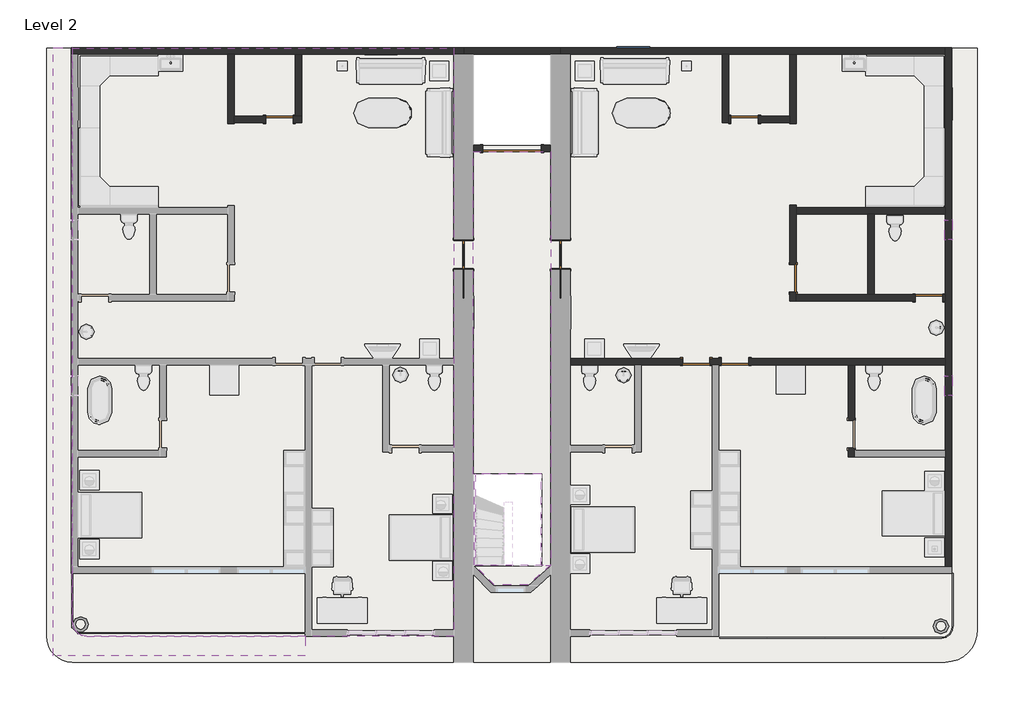
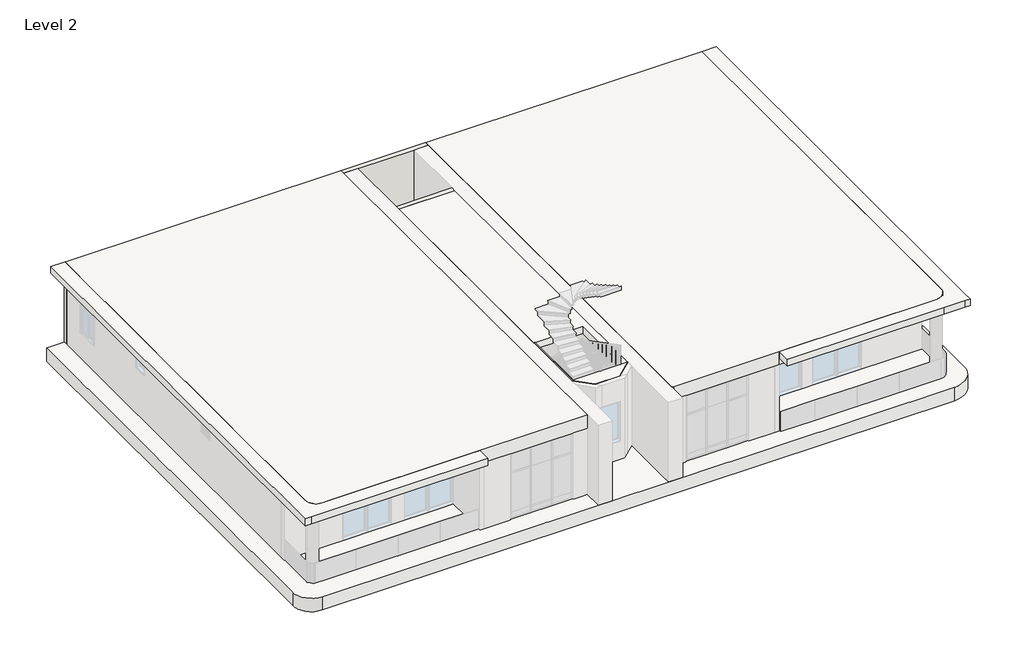
# One storey, part 3 of 5: 17 walls, 9 doors, 5 windows, 4 slabs, 1 roof.
"""IFC4 building model written with IfcOpenShell, lengths in millimetres."""

from ifc_helpers import new_model, si_unit, point, frame, frame_2d, origin, place, context, project, spatial, polyline, circle_curve, trimmed, segment, composite_curve, outline, extrude, faceted_brep, transform, mapped, element, save
from components import door_4726f842, door_ede55593, door_2703ae13, door_10fd3a06, window_0038ecf3, window_54100e87

model = new_model("IFC4")

# Units and contexts
model_context = context("Model", 3, world=origin())
ifc_project = project(units=[si_unit("LENGTHUNIT", "METRE", prefix="MILLI")], contexts=[model_context])

# Site, building, storey
site = spatial("IfcSite", under=ifc_project)
building = spatial("IfcBuilding", under=site)
storey = spatial("IfcBuildingStorey", under=building, Name="Level 2", Elevation=3657.6)

# Doors
placement = place(None, origin())
door_shape = door_4726f842(model_context)
element("IfcDoor", 1, ObjectType="Door-Double-Flush_Panel-Double-Acting : 72\" x 84\"", at=placement, inside=storey, context=model_context, shape_type="MappedRepresentation", body=[
    mapped(door_shape, transform((-4793.1987704, 8549.6758558, 3657.6), x_axis=(-1.0, 0.0, 0.0), y_axis=(0.0, -1.0, 0.0), z_axis=(0.0, 0.0, 1.0))),
])
door_2_shape = door_ede55593(model_context)
element("IfcDoor", 2, ObjectType="Door-Interior-Single-Pocket-2_Panel-Wood : 36\" x 96\"", at=placement, inside=storey, context=model_context, shape_type="MappedRepresentation", body=[
    mapped(door_2_shape, transform((-6317.1987704, 5196.8758558, 3657.6), x_axis=(0.0, -1.0, 0.0), y_axis=(1.0, 0.0, 0.0), z_axis=(0.0, 0.0, 1.0))),
])
element("IfcDoor", 3, ObjectType="Door-Interior-Single-Pocket-2_Panel-Wood : 36\" x 96\"", at=placement, inside=storey, context=model_context, shape_type="MappedRepresentation", body=[
    mapped(door_2_shape, transform((-3269.1987704, 5196.8758558, 3657.6), x_axis=(0.0, -1.0, 0.0), y_axis=(1.0, 0.0, 0.0), z_axis=(0.0, 0.0, 1.0))),
])
door_3_shape = door_2703ae13(model_context)
element("IfcDoor", 4, ObjectType="Door-Single-Panel.0001 : 34\" x 80\"", at=placement, inside=storey, context=model_context, shape_type="MappedRepresentation", body=[
    mapped(door_3_shape, transform((998.0012296, 1844.0758558, 3657.6), x_axis=(1.0, 0.0, 0.0), y_axis=(0.0, 1.0, 0.0), z_axis=(0.0, 0.0, 1.0))),
])
element("IfcDoor", 5, ObjectType="Door-Single-Panel.0001 : 34\" x 80\"", at=placement, inside=storey, context=model_context, shape_type="MappedRepresentation", body=[
    mapped(door_3_shape, transform((2522.0012296, 9464.0758558, 3657.6), x_axis=(-1.0, 0.0, 0.0), y_axis=(0.0, -1.0, 0.0), z_axis=(0.0, 0.0, 1.0))),
])
door_4_shape = door_10fd3a06(model_context)
element("IfcDoor", 6, ObjectType="Door-Single-Panel.0001 : 34\" x 80\"", at=placement, inside=storey, context=model_context, shape_type="MappedRepresentation", body=[
    mapped(door_4_shape, transform((-12108.3987704, 9464.0758558, 3657.6), x_axis=(1.0, 0.0, 0.0), y_axis=(0.0, 1.0, 0.0), z_axis=(0.0, 0.0, 1.0))),
])
element("IfcDoor", 7, ObjectType="Door-Single-Panel.0001 : 34\" x 80\"", at=placement, inside=storey, context=model_context, shape_type="MappedRepresentation", body=[
    mapped(door_4_shape, transform((2217.2012296, 1844.0758558, 3657.6), x_axis=(-1.0, 0.0, 0.0), y_axis=(0.0, -1.0, 0.0), z_axis=(0.0, 0.0, 1.0))),
])
element("IfcDoor", 8, ObjectType="Door-Single-Panel.0001 : 34\" x 80\"", at=placement, inside=storey, context=model_context, shape_type="MappedRepresentation", body=[
    mapped(door_4_shape, transform((8313.2012296, 3850.6758558, 3657.6), x_axis=(1.0, 0.0, 0.0), y_axis=(0.0, 1.0, 0.0), z_axis=(0.0, 0.0, 1.0))),
])
element("IfcDoor", 9, ObjectType="Door-Single-Panel.0001 : 34\" x 80\"", at=placement, inside=storey, context=model_context, shape_type="MappedRepresentation", body=[
    mapped(door_4_shape, transform((4046.0012296, 4460.2758558, 3657.6), x_axis=(0.0, -1.0, 0.0), y_axis=(1.0, 0.0, 0.0), z_axis=(0.0, 0.0, 1.0))),
])

# Roof
element("IfcRoof", 10, ObjectType="Generic - 2' white 2", at=placement, inside=storey, context=model_context, shape_type="SweptSolid", body=[
    extrude(outline(composite_curve([segment(polyline([(-19423.5987704, 11699.2758558), (9837.2012296, 11699.2758558), (9837.2012296, -6588.7241442)]), True, "CONTINUOUS"), segment(trimmed(circle_curve(frame_2d((8821.2012296, -6588.7241442)), 1016.0), [point((9837.2012296, -6588.7241442))], [point((8821.2012296, -7604.7241442))], False, "CARTESIAN"), True, "CONTINUOUS"), segment(polyline([(8821.2012296, -7604.7241442), (-18610.7987704, -7604.7241442)]), True, "CONTINUOUS"), segment(trimmed(circle_curve(frame_2d((-18610.7987704, -6791.9241442)), 812.8), [point((-18610.7987704, -7604.7241442))], [point((-19423.5987704, -6791.9241442))], False, "CARTESIAN"), True, "CONTINUOUS"), segment(polyline([(-19423.5987704, -6791.9241442), (-19423.5987704, 11699.2758558)]), True, "CONTINUOUS")], self_intersect=False), holes=[polyline([(-6012.3987704, -4575.7741442), (-3853.3987704, -4575.7741442), (-3853.3987704, -1686.5241442), (-6012.3987704, -1686.5241442), (-6012.3987704, -4575.7741442)]), polyline([(-6012.3987704, 8651.2758558), (-3573.9987704, 8651.2758558), (-3573.9987704, 11521.4758558), (-6012.3987704, 11521.4758558), (-6012.3987704, 8651.2758558)])]), frame((0.0, 0.0, 3048.0), z_axis=(0.0, 0.0, 1.0), x_axis=(1.0, 0.0, 0.0)), (0.0, 0.0, 1.0), 609.6),
])

# Slabs
element("IfcSlab", 11, ObjectType="Generic - 12\" cream", at=placement, inside=storey, context=model_context, shape_type="SweptSolid", body=[
    extrude(outline(composite_curve([segment(polyline([(-6621.9987704, 11699.2758558), (-6621.9987704, -6791.9241442), (-11295.5987704, -6791.9241442), (-18153.5987704, -6791.9241442)]), True, "CONTINUOUS"), segment(trimmed(circle_curve(frame_2d((-18153.5987704, -6334.7241442)), 457.2), [point((-18153.5987704, -6791.9241442))], [point((-18610.7987704, -6334.7241442))], False, "CARTESIAN"), True, "CONTINUOUS"), segment(polyline([(-18610.7987704, -6334.7241442), (-18610.7987704, 11699.2758558), (-6621.9987704, 11699.2758558)]), True, "CONTINUOUS")], self_intersect=False)), frame((0.0, 0.0, 6705.6), z_axis=(0.0, 0.0, 1.0), x_axis=(1.0, 0.0, 0.0)), (0.0, 0.0, 1.0), 609.6),
    extrude(outline(composite_curve([segment(trimmed(circle_curve(frame_2d((8511.8043381, -6277.3874522)), 514.536692), [point((9024.4012296, -6322.0241442))], [point((8511.8043381, -6791.9241442))], False, "CARTESIAN"), True, "CONTINUOUS"), segment(polyline([(8511.8043381, -6791.9241442), (1709.2012296, -6791.9241442), (-2862.7987704, -6791.9241442), (-2964.3987704, -6791.9241442), (-2964.3987704, 11699.2758558), (9024.4012296, 11699.2758558), (9024.4012296, -6322.0241442)]), True, "CONTINUOUS")], self_intersect=False)), frame((0.0, 0.0, 6705.6), z_axis=(0.0, 0.0, 1.0), x_axis=(1.0, 0.0, 0.0)), (0.0, 0.0, 1.0), 609.6),
])
element("IfcSlab", 12, ObjectType="Generic - 12\" white", at=placement, inside=storey, context=model_context, shape_type="SweptSolid", body=[
    extrude(outline(composite_curve([segment(polyline([(9634.0012296, 11699.2758558), (9634.0012296, -6931.6241442), (9634.0012296, -7401.5241442), (9430.8012296, -7401.5241442), (8511.8043381, -7401.5241442), (1709.2012296, -7401.5241442), (1709.2012296, -6791.9241442), (8511.8043381, -6791.9241442)]), True, "CONTINUOUS"), segment(trimmed(circle_curve(frame_2d((8511.8043381, -6277.3874522)), 514.536692), [point((8511.8043381, -6791.9241442))], [point((9024.4012296, -6322.0241442))], True, "CARTESIAN"), True, "CONTINUOUS"), segment(polyline([(9024.4012296, -6322.0241442), (9024.4012296, 11699.2758558), (9634.0012296, 11699.2758558)]), True, "CONTINUOUS")], self_intersect=False)), frame((0.0, 0.0, 7010.4), z_axis=(0.0, 0.0, 1.0), x_axis=(1.0, 0.0, 0.0)), (0.0, 0.0, 1.0), 304.8),
    extrude(outline(composite_curve([segment(polyline([(-18610.7987704, 11724.6758558), (-18610.7987704, -6334.7241442)]), True, "CONTINUOUS"), segment(trimmed(circle_curve(frame_2d((-18153.5987704, -6334.7241442)), 457.2), [point((-18610.7987704, -6334.7241442))], [point((-18153.5987704, -6791.9241442))], True, "CARTESIAN"), True, "CONTINUOUS"), segment(polyline([(-18153.5987704, -6791.9241442), (-11295.5987704, -6791.9241442), (-11295.5987704, -7401.5241442), (-18966.3987704, -7401.5241442), (-19220.3987704, -7401.5241442), (-19220.3987704, 11724.6758558), (-18610.7987704, 11724.6758558)]), True, "CONTINUOUS")], self_intersect=False)), frame((0.0, 0.0, 7010.4), z_axis=(0.0, 0.0, 1.0), x_axis=(1.0, 0.0, 0.0)), (0.0, 0.0, 1.0), 304.8),
])
element("IfcSlab", 13, ObjectType="Generic - 12\" white", at=placement, inside=storey, context=model_context, shape_type="SweptSolid", body=[
    extrude(outline(polyline([(-3573.9987704, 8448.0758558), (-3573.9987704, -1691.5549149), (-3573.9987704, -4572.9908503), (-3878.7987704, -4572.9908503), (-3878.7987704, -1691.5549149), (-6012.3987704, -1691.5549149), (-6012.3987704, 8448.0758558), (-3573.9987704, 8448.0758558)])), frame((0.0, 0.0, 7010.4), z_axis=(0.0, 0.0, 1.0), x_axis=(1.0, 0.0, 0.0)), (0.0, 0.0, 1.0), 304.8),
])
element("IfcSlab", 14, ObjectType="Generic - 12\" white", at=placement, inside=storey, context=model_context, shape_type="SweptSolid", body=[
    extrude(outline(polyline([(-5940.8822214, -1691.5549149), (-5940.8822214, -4554.2130548), (-3578.6822214, -4554.2130548), (-4280.0806614, -5179.7242605), (-5346.8806614, -5179.7242605), (-5975.4985898, -4551.106332), (-5975.4985898, -1691.5549149), (-5940.8822214, -1691.5549149)])), frame((0.0, 0.0, 7010.4), z_axis=(0.0, 0.0, 1.0), x_axis=(1.0, 0.0, 0.0)), (0.0, 0.0, 1.0), 304.8),
])

# Walls
element("IfcWall", 15, ObjectType="Generic - 8\" cream", at=placement, inside=storey, context=model_context, shape_type="Brep", body=[
    faceted_brep([(-18648.8987704, 11521.4758558, 3657.6), (-18445.6987704, 11521.4758558, 3657.6), (-13733.9987704, 11521.4758558, 3657.6), (-13530.7987704, 11521.4758558, 3657.6), (-11600.3987704, 11521.4758558, 3657.6), (-11397.1987704, 11521.4758558, 3657.6), (-6621.9987704, 11521.4758558, 3657.6), (-6317.1987704, 11521.4758558, 3657.6), (-6317.1987704, 11521.4758558, 6705.6), (-6621.9987704, 11521.4758558, 6705.6), (-11397.1987704, 11521.4758558, 6705.6), (-11600.3987704, 11521.4758558, 6705.6), (-13530.7987704, 11521.4758558, 6705.6), (-13733.9987704, 11521.4758558, 6705.6), (-18445.6987704, 11521.4758558, 6705.6), (-18648.8987704, 11521.4758558, 6705.6), (-8450.7987704, 11521.4758558, 6096.0), (-8450.7987704, 11521.4758558, 4876.8), (-9365.1987704, 11521.4758558, 4876.8), (-9365.1987704, 11521.4758558, 6096.0), (-6317.1987704, 11724.6758558, 3657.6), (-18648.8987704, 11724.6758558, 3657.6), (-18648.8987704, 11724.6758558, 6705.6), (-6621.9987704, 11724.6758558, 6705.6), (-6317.1987704, 11724.6758558, 6705.6), (-8450.7987704, 11724.6758558, 4876.8), (-8450.7987704, 11724.6758558, 6096.0), (-9365.1987704, 11724.6758558, 6096.0), (-9365.1987704, 11724.6758558, 4876.8)], [[[0, 1, 2, 3, 4, 5, 6, 7, 8, 9, 10, 11, 12, 13, 14, 15], [16, 17, 18, 19]], [[20, 21, 22, 23, 24], [25, 26, 27, 28]], [[7, 6, 5, 4, 3, 2, 1, 0, 21, 20]], [[8, 7, 20, 24]], [[15, 14, 13, 12, 11, 10, 9, 8, 24, 23, 22]], [[0, 15, 22, 21]], [[16, 26, 25, 17]], [[17, 25, 28, 18]], [[18, 28, 27, 19]], [[26, 16, 19, 27]]]),
])
element("IfcWall", 16, ObjectType="Generic - 8\" cream", at=placement, inside=storey, context=model_context, shape_type="Brep", body=[
    faceted_brep([(8821.2012296, 11724.6758558, 3657.6), (8821.2012296, 11521.4758558, 3657.6), (8821.2012296, 6695.4758558, 3657.6), (8821.2012296, 6492.2758558, 3657.6), (8821.2012296, 3952.2758558, 3657.6), (8821.2012296, 3749.0758558, 3657.6), (8821.2012296, 1945.6758558, 3657.6), (8821.2012296, 1742.4758558, 3657.6), (8821.2012296, -949.9241442, 3657.6), (8821.2012296, -1153.1241442, 3657.6), (8821.2012296, -4607.5241442, 3657.6), (8821.2012296, -4607.5241442, 6705.6), (8821.2012296, -1153.1241442, 6705.6), (8821.2012296, -949.9241442, 6705.6), (8821.2012296, 1742.4758558, 6705.6), (8821.2012296, 1945.6758558, 6705.6), (8821.2012296, 3749.0758558, 6705.6), (8821.2012296, 3952.2758558, 6705.6), (8821.2012296, 6492.2758558, 6705.6), (8821.2012296, 6695.4758558, 6705.6), (8821.2012296, 11521.4758558, 6705.6), (8821.2012296, 11724.6758558, 6705.6), (8821.2012296, 10403.8758558, 4876.8), (8821.2012296, 10403.8758558, 6096.0), (8821.2012296, 9489.4758558, 6096.0), (8821.2012296, 9489.4758558, 4876.8), (8821.2012296, 777.2758558, 6400.8), (8821.2012296, 777.2758558, 5791.2), (8821.2012296, 1386.8758558, 5791.2), (8821.2012296, 1386.8758558, 6400.8), (8821.2012296, 6289.0758558, 5791.2), (8821.2012296, 6289.0758558, 6400.8), (8821.2012296, 5679.4758558, 6400.8), (8821.2012296, 5679.4758558, 5791.2), (9024.4012296, -4607.5241442, 3657.6), (9024.4012296, 11724.6758558, 3657.6), (9024.4012296, 11724.6758558, 6705.6), (9024.4012296, -4607.5241442, 6705.6), (9024.4012296, 10403.8758558, 6096.0), (9024.4012296, 10403.8758558, 4876.8), (9024.4012296, 9489.4758558, 4876.8), (9024.4012296, 9489.4758558, 6096.0), (9024.4012296, 777.2758558, 5791.2), (9024.4012296, 777.2758558, 6400.8), (9024.4012296, 1386.8758558, 6400.8), (9024.4012296, 1386.8758558, 5791.2), (9024.4012296, 6289.0758558, 6400.8), (9024.4012296, 6289.0758558, 5791.2), (9024.4012296, 5679.4758558, 5791.2), (9024.4012296, 5679.4758558, 6400.8)], [[[0, 1, 2, 3, 4, 5, 6, 7, 8, 9, 10, 11, 12, 13, 14, 15, 16, 17, 18, 19, 20, 21], [22, 23, 24, 25], [26, 27, 28, 29], [30, 31, 32, 33]], [[34, 35, 36, 37], [38, 39, 40, 41], [42, 43, 44, 45], [46, 47, 48, 49]], [[10, 9, 8, 7, 6, 5, 4, 3, 2, 1, 0, 35, 34]], [[21, 20, 19, 18, 17, 16, 15, 14, 13, 12, 11, 37, 36]], [[0, 21, 36, 35]], [[11, 10, 34, 37]], [[39, 38, 23, 22]], [[40, 39, 22, 25]], [[41, 40, 25, 24]], [[38, 41, 24, 23]], [[26, 43, 42, 27]], [[27, 42, 45, 28]], [[28, 45, 44, 29]], [[43, 26, 29, 44]], [[46, 31, 30, 47]], [[47, 30, 33, 48]], [[48, 33, 32, 49]], [[31, 46, 49, 32]]]),
])
element("IfcWall", 17, ObjectType="Generic - 8\" cream", at=placement, inside=storey, context=model_context, shape_type="Brep", body=[
    faceted_brep([(8821.2012296, 1742.4758558, 6705.6), (5976.4012296, 1742.4758558, 6705.6), (5773.2012296, 1742.4758558, 6705.6), (1709.2012296, 1742.4758558, 6705.6), (1506.0012296, 1742.4758558, 6705.6), (-729.1987704, 1742.4758558, 6705.6), (-932.3987704, 1742.4758558, 6705.6), (-2964.3987704, 1742.4758558, 6705.6), (-2964.3987704, 1742.4758558, 3657.6), (-932.3987704, 1742.4758558, 3657.6), (-729.1987704, 1742.4758558, 3657.6), (566.2012296, 1742.4758558, 3657.6), (566.2012296, 1742.4758558, 5689.6), (1429.8012296, 1742.4758558, 5689.6), (1429.8012296, 1742.4758558, 3657.6), (1506.0012296, 1742.4758558, 3657.6), (1709.2012296, 1742.4758558, 3657.6), (1785.4012296, 1742.4758558, 3657.6), (1785.4012296, 1742.4758558, 5689.6), (2649.0012296, 1742.4758558, 5689.6), (2649.0012296, 1742.4758558, 3657.6), (5773.2012296, 1742.4758558, 3657.6), (5976.4012296, 1742.4758558, 3657.6), (8821.2012296, 1742.4758558, 3657.6), (-2964.3987704, 1945.6758558, 6705.6), (8821.2012296, 1945.6758558, 6705.6), (8821.2012296, 1945.6758558, 3657.6), (2649.0012296, 1945.6758558, 3657.6), (2649.0012296, 1945.6758558, 5689.6), (1785.4012296, 1945.6758558, 5689.6), (1785.4012296, 1945.6758558, 3657.6), (1429.8012296, 1945.6758558, 3657.6), (1429.8012296, 1945.6758558, 5689.6), (566.2012296, 1945.6758558, 5689.6), (566.2012296, 1945.6758558, 3657.6), (-2964.3987704, 1945.6758558, 3657.6)], [[[0, 1, 2, 3, 4, 5, 6, 7, 8, 9, 10, 11, 12, 13, 14, 15, 16, 17, 18, 19, 20, 21, 22, 23]], [[24, 25, 26, 27, 28, 29, 30, 31, 32, 33, 34, 35]], [[8, 35, 34, 11, 10, 9]], [[26, 23, 22, 21, 20, 27]], [[14, 31, 30, 17, 16, 15]], [[7, 6, 5, 4, 3, 2, 1, 0, 25, 24]], [[0, 23, 26, 25]], [[8, 7, 24, 35]], [[13, 32, 31, 14]], [[32, 13, 12, 33]], [[33, 12, 11, 34]], [[29, 18, 17, 30]], [[18, 29, 28, 19]], [[19, 28, 27, 20]]]),
])
element("IfcWall", 18, ObjectType="Generic - 8\" cream", at=placement, inside=storey, context=model_context, shape_type="Brep", body=[
    faceted_brep([(-13733.9987704, 11521.4758558, 3657.6), (-13733.9987704, 9337.0758558, 3657.6), (-13733.9987704, 9337.0758558, 6705.6), (-13733.9987704, 11521.4758558, 6705.6), (-13530.7987704, 11521.4758558, 3657.6), (-13530.7987704, 11521.4758558, 6705.6), (-13530.7987704, 9565.6758558, 6705.6), (-13530.7987704, 9362.4758558, 6705.6), (-13530.7987704, 9337.0758558, 6705.6), (-13530.7987704, 9337.0758558, 3657.6), (-13530.7987704, 9362.4758558, 3657.6), (-13530.7987704, 9565.6758558, 3657.6)], [[[0, 1, 2, 3]], [[4, 5, 6, 7, 8, 9, 10, 11]], [[1, 0, 4, 11, 10, 9]], [[2, 1, 9, 8]], [[3, 2, 8, 7, 6, 5]], [[0, 3, 5, 4]]]),
])
element("IfcWall", 19, ObjectType="Generic - 8\" cream", at=placement, inside=storey, context=model_context, shape_type="Brep", body=[
    faceted_brep([(-11397.1987704, 9362.4758558, 6705.6), (-13530.7987704, 9362.4758558, 6705.6), (-13530.7987704, 9362.4758558, 3657.6), (-12540.1987704, 9362.4758558, 3657.6), (-12540.1987704, 9362.4758558, 5689.6), (-11676.5987704, 9362.4758558, 5689.6), (-11676.5987704, 9362.4758558, 3657.6), (-11397.1987704, 9362.4758558, 3657.6), (-13530.7987704, 9565.6758558, 6705.6), (-11600.3987704, 9565.6758558, 6705.6), (-11397.1987704, 9565.6758558, 6705.6), (-11397.1987704, 9565.6758558, 3657.6), (-11600.3987704, 9565.6758558, 3657.6), (-11676.5987704, 9565.6758558, 3657.6), (-11676.5987704, 9565.6758558, 5689.6), (-12540.1987704, 9565.6758558, 5689.6), (-12540.1987704, 9565.6758558, 3657.6), (-13530.7987704, 9565.6758558, 3657.6)], [[[0, 1, 2, 3, 4, 5, 6, 7]], [[8, 9, 10, 11, 12, 13, 14, 15, 16, 17]], [[2, 17, 16, 3]], [[11, 7, 6, 13, 12]], [[1, 0, 10, 9, 8]], [[2, 1, 8, 17]], [[0, 7, 11, 10]], [[5, 14, 13, 6]], [[14, 5, 4, 15]], [[15, 4, 3, 16]]]),
])
element("IfcWall", 20, ObjectType="Generic - 8\" cream", at=placement, inside=storey, context=model_context, shape_type="SweptSolid", body=[
    extrude(outline(polyline([(-11397.1987704, 11521.4758558), (-11397.1987704, 9565.6758558), (-11600.3987704, 9565.6758558), (-11600.3987704, 11521.4758558), (-11397.1987704, 11521.4758558)])), frame((0.0, 0.0, 3657.6), z_axis=(0.0, 0.0, 1.0), x_axis=(1.0, 0.0, 0.0)), (0.0, 0.0, 1.0), 3048.0),
])
element("IfcWall", 21, ObjectType="Generic - 8\" cream", at=placement, inside=storey, context=model_context, shape_type="Brep", body=[
    faceted_brep([(3944.4012296, 11521.4758558, 3657.6), (3944.4012296, 9565.6758558, 3657.6), (3944.4012296, 9362.4758558, 3657.6), (3944.4012296, 9337.0758558, 3657.6), (3944.4012296, 9337.0758558, 6705.6), (3944.4012296, 9362.4758558, 6705.6), (3944.4012296, 9565.6758558, 6705.6), (3944.4012296, 11521.4758558, 6705.6), (4147.6012296, 11521.4758558, 3657.6), (4147.6012296, 11521.4758558, 6705.6), (4147.6012296, 9337.0758558, 6705.6), (4147.6012296, 9337.0758558, 3657.6)], [[[0, 1, 2, 3, 4, 5, 6, 7]], [[8, 9, 10, 11]], [[3, 2, 1, 0, 8, 11]], [[4, 3, 11, 10]], [[7, 6, 5, 4, 10, 9]], [[0, 7, 9, 8]]]),
])
element("IfcWall", 22, ObjectType="Generic - 8\" cream", at=placement, inside=storey, context=model_context, shape_type="Brep", body=[
    faceted_brep([(4147.6012296, 6492.2758558, 3657.6), (6382.8012296, 6492.2758558, 3657.6), (6586.0012296, 6492.2758558, 3657.6), (8821.2012296, 6492.2758558, 3657.6), (8821.2012296, 6492.2758558, 6705.6), (6586.0012296, 6492.2758558, 6705.6), (6382.8012296, 6492.2758558, 6705.6), (4147.6012296, 6492.2758558, 6705.6), (4147.6012296, 6695.4758558, 3657.6), (4147.6012296, 6695.4758558, 6705.6), (8821.2012296, 6695.4758558, 6705.6), (8821.2012296, 6695.4758558, 3657.6)], [[[0, 1, 2, 3, 4, 5, 6, 7]], [[8, 9, 10, 11]], [[3, 2, 1, 0, 8, 11]], [[7, 6, 5, 4, 10, 9]], [[0, 7, 9, 8]], [[4, 3, 11, 10]]]),
])
element("IfcWall", 23, ObjectType="Generic - 8\" cream", at=placement, inside=storey, context=model_context, shape_type="Brep", body=[
    faceted_brep([(8821.2012296, 3749.0758558, 6705.6), (4147.6012296, 3749.0758558, 6705.6), (4147.6012296, 3749.0758558, 3657.6), (7881.4012296, 3749.0758558, 3657.6), (7881.4012296, 3749.0758558, 5689.6), (8745.0012296, 3749.0758558, 5689.6), (8745.0012296, 3749.0758558, 3657.6), (8821.2012296, 3749.0758558, 3657.6), (4147.6012296, 3952.2758558, 6705.6), (6382.8012296, 3952.2758558, 6705.6), (6586.0012296, 3952.2758558, 6705.6), (8821.2012296, 3952.2758558, 6705.6), (8821.2012296, 3952.2758558, 3657.6), (8745.0012296, 3952.2758558, 3657.6), (8745.0012296, 3952.2758558, 5689.6), (7881.4012296, 3952.2758558, 5689.6), (7881.4012296, 3952.2758558, 3657.6), (6586.0012296, 3952.2758558, 3657.6), (6382.8012296, 3952.2758558, 3657.6), (4147.6012296, 3952.2758558, 3657.6)], [[[0, 1, 2, 3, 4, 5, 6, 7]], [[8, 9, 10, 11, 12, 13, 14, 15, 16, 17, 18, 19]], [[2, 19, 18, 17, 16, 3]], [[12, 7, 6, 13]], [[1, 0, 11, 10, 9, 8]], [[2, 1, 8, 19]], [[0, 7, 12, 11]], [[5, 14, 13, 6]], [[14, 5, 4, 15]], [[15, 4, 3, 16]]]),
])
element("IfcWall", 24, ObjectType="Generic - 8\" cream", at=placement, inside=storey, context=model_context, shape_type="SweptSolid", body=[
    extrude(outline(polyline([(6705.6, 3944.4012296), (6705.6, 2014.0012296), (3657.6, 2014.0012296), (3657.6, 2090.2012296), (5689.6, 2090.2012296), (5689.6, 2953.8012296), (3657.6, 2953.8012296), (3657.6, 3944.4012296), (6705.6, 3944.4012296)])), frame((0.0, 9362.4758558, 0.0), z_axis=(0.0, 1.0, 0.0), x_axis=(0.0, 0.0, 1.0)), (0.0, 0.0, 1.0), 203.2),
])
element("IfcWall", 25, ObjectType="Generic - 8\" cream", at=placement, inside=storey, context=model_context, shape_type="Brep", body=[
    faceted_brep([(5773.2012296, -1153.1241442, 6705.6), (5773.2012296, 1742.4758558, 6705.6), (5773.2012296, 1742.4758558, 3657.6), (5773.2012296, -10.1241442, 3657.6), (5773.2012296, -10.1241442, 5689.6), (5773.2012296, -873.7241442, 5689.6), (5773.2012296, -873.7241442, 3657.6), (5773.2012296, -1153.1241442, 3657.6), (5976.4012296, 1742.4758558, 6705.6), (5976.4012296, -949.9241442, 6705.6), (5976.4012296, -1153.1241442, 6705.6), (5976.4012296, -1153.1241442, 3657.6), (5976.4012296, -949.9241442, 3657.6), (5976.4012296, -873.7241442, 3657.6), (5976.4012296, -873.7241442, 5689.6), (5976.4012296, -10.1241442, 5689.6), (5976.4012296, -10.1241442, 3657.6), (5976.4012296, 1742.4758558, 3657.6)], [[[0, 1, 2, 3, 4, 5, 6, 7]], [[8, 9, 10, 11, 12, 13, 14, 15, 16, 17]], [[2, 17, 16, 3]], [[11, 7, 6, 13, 12]], [[1, 0, 10, 9, 8]], [[2, 1, 8, 17]], [[0, 7, 11, 10]], [[5, 14, 13, 6]], [[14, 5, 4, 15]], [[15, 4, 3, 16]]]),
])
element("IfcWall", 26, ObjectType="Generic - 8\" cream", at=placement, inside=storey, context=model_context, shape_type="SweptSolid", body=[
    extrude(outline(polyline([(6382.8012296, 3952.2758558), (6382.8012296, 6492.2758558), (6586.0012296, 6492.2758558), (6586.0012296, 3952.2758558), (6382.8012296, 3952.2758558)])), frame((0.0, 0.0, 3657.6), z_axis=(0.0, 0.0, 1.0), x_axis=(1.0, 0.0, 0.0)), (0.0, 0.0, 1.0), 3048.0),
])
element("IfcWall", 27, ObjectType="Generic - 8\" cream", at=placement, inside=storey, context=model_context, shape_type="SweptSolid", body=[
    extrude(outline(polyline([(7315.2, -3573.9987704), (7315.2, -6012.3987704), (3657.6, -6012.3987704), (3657.6, -5707.5987704), (5791.2, -5707.5987704), (5791.2, -3878.7987704), (3657.6, -3878.7987704), (3657.6, -3573.9987704), (7315.2, -3573.9987704)])), frame((0.0, 8448.0758558, 0.0), z_axis=(0.0, 1.0, 0.0), x_axis=(0.0, 0.0, 1.0)), (0.0, 0.0, 1.0), 203.2),
])
element("IfcWall", 28, ObjectType="Generic - 8\" cream", at=placement, inside=storey, context=model_context, shape_type="Brep", body=[
    faceted_brep([(3944.4012296, 3749.0758558, 6705.6), (3944.4012296, 6771.6758558, 6705.6), (3944.4012296, 6771.6758558, 3657.6), (3944.4012296, 4892.0758558, 3657.6), (3944.4012296, 4892.0758558, 5689.6), (3944.4012296, 4028.4758558, 5689.6), (3944.4012296, 4028.4758558, 3657.6), (3944.4012296, 3749.0758558, 3657.6), (4147.6012296, 6771.6758558, 6705.6), (4147.6012296, 6695.4758558, 6705.6), (4147.6012296, 6492.2758558, 6705.6), (4147.6012296, 3952.2758558, 6705.6), (4147.6012296, 3749.0758558, 6705.6), (4147.6012296, 3749.0758558, 3657.6), (4147.6012296, 3952.2758558, 3657.6), (4147.6012296, 4028.4758558, 3657.6), (4147.6012296, 4028.4758558, 5689.6), (4147.6012296, 4892.0758558, 5689.6), (4147.6012296, 4892.0758558, 3657.6), (4147.6012296, 6492.2758558, 3657.6), (4147.6012296, 6695.4758558, 3657.6), (4147.6012296, 6771.6758558, 3657.6)], [[[0, 1, 2, 3, 4, 5, 6, 7]], [[8, 9, 10, 11, 12, 13, 14, 15, 16, 17, 18, 19, 20, 21]], [[2, 21, 20, 19, 18, 3]], [[13, 7, 6, 15, 14]], [[1, 0, 12, 11, 10, 9, 8]], [[2, 1, 8, 21]], [[0, 7, 13, 12]], [[5, 16, 15, 6]], [[16, 5, 4, 17]], [[17, 4, 3, 18]]]),
])
element("IfcWall", 29, ObjectType="Generic - 8\" cream", at=placement, inside=storey, context=model_context, shape_type="Brep", body=[
    faceted_brep([(-6317.1987704, 11521.4758558, 3657.6), (-6012.3987704, 11521.4758558, 3657.6), (-3573.9987704, 11521.4758558, 3657.6), (-3269.1987704, 11521.4758558, 3657.6), (-3269.1987704, 11521.4758558, 6705.6), (-2964.3987704, 11521.4758558, 6705.6), (-2964.3987704, 11521.4758558, 7315.2), (-3573.9987704, 11521.4758558, 7315.2), (-6012.3987704, 11521.4758558, 7315.2), (-6621.9987704, 11521.4758558, 7315.2), (-6621.9987704, 11521.4758558, 6705.6), (-6317.1987704, 11521.4758558, 6705.6), (-6317.1987704, 11724.6758558, 3657.6), (-6317.1987704, 11724.6758558, 6705.6), (-6621.9987704, 11724.6758558, 6705.6), (-6621.9987704, 11724.6758558, 7315.2), (-2964.3987704, 11724.6758558, 7315.2), (-2964.3987704, 11724.6758558, 6705.6), (-3269.1987704, 11724.6758558, 6705.6), (-3269.1987704, 11724.6758558, 3657.6)], [[[0, 1, 2, 3, 4, 5, 6, 7, 8, 9, 10, 11]], [[12, 13, 14, 15, 16, 17, 18, 19]], [[3, 2, 1, 0, 12, 19]], [[9, 8, 7, 6, 16, 15]], [[0, 11, 13, 12]], [[10, 14, 13, 11]], [[10, 9, 15, 14]], [[4, 3, 19, 18]], [[17, 5, 4, 18]], [[6, 5, 17, 16]]]),
])
element("IfcWall", 30, ObjectType="Generic - 8\" cream", at=placement, inside=storey, context=model_context, shape_type="Brep", body=[
    faceted_brep([(-3269.1987704, 11521.4758558, 3657.6), (-2964.3987704, 11521.4758558, 3657.6), (1810.8012296, 11521.4758558, 3657.6), (2014.0012296, 11521.4758558, 3657.6), (3944.4012296, 11521.4758558, 3657.6), (4147.6012296, 11521.4758558, 3657.6), (8821.2012296, 11521.4758558, 3657.6), (8821.2012296, 11521.4758558, 6705.6), (4147.6012296, 11521.4758558, 6705.6), (3944.4012296, 11521.4758558, 6705.6), (2014.0012296, 11521.4758558, 6705.6), (1810.8012296, 11521.4758558, 6705.6), (-2964.3987704, 11521.4758558, 6705.6), (-3269.1987704, 11521.4758558, 6705.6), (-1440.3987704, 11521.4758558, 6096.0), (-525.9987704, 11521.4758558, 6096.0), (-525.9987704, 11521.4758558, 4876.8), (-1440.3987704, 11521.4758558, 4876.8), (-3269.1987704, 11724.6758558, 3657.6), (-3269.1987704, 11724.6758558, 6705.6), (-2964.3987704, 11724.6758558, 6705.6), (8821.2012296, 11724.6758558, 6705.6), (8821.2012296, 11724.6758558, 3657.6), (-1440.3987704, 11724.6758558, 6096.0), (-1440.3987704, 11724.6758558, 4876.8), (-525.9987704, 11724.6758558, 4876.8), (-525.9987704, 11724.6758558, 6096.0)], [[[0, 1, 2, 3, 4, 5, 6, 7, 8, 9, 10, 11, 12, 13], [14, 15, 16, 17]], [[18, 19, 20, 21, 22], [23, 24, 25, 26]], [[6, 5, 4, 3, 2, 1, 0, 18, 22]], [[13, 12, 11, 10, 9, 8, 7, 21, 20, 19]], [[0, 13, 19, 18]], [[7, 6, 22, 21]], [[23, 26, 15, 14]], [[26, 25, 16, 15]], [[25, 24, 17, 16]], [[24, 23, 14, 17]]]),
])
element("IfcWall", 31, ObjectType="Generic - 8\" white", at=placement, inside=storey, context=model_context, shape_type="Brep", body=[
    faceted_brep([(1810.8012296, 11521.4758558, 3657.6), (1810.8012296, 9362.4758558, 3657.6), (1810.8012296, 9362.4758558, 6705.6), (1810.8012296, 11521.4758558, 6705.6), (2014.0012296, 11521.4758558, 3657.6), (2014.0012296, 11521.4758558, 6705.6), (2014.0012296, 9565.6758558, 6705.6), (2014.0012296, 9362.4758558, 6705.6), (2014.0012296, 9362.4758558, 3657.6), (2014.0012296, 9565.6758558, 3657.6)], [[[0, 1, 2, 3]], [[4, 5, 6, 7, 8, 9]], [[1, 0, 4, 9, 8]], [[3, 2, 7, 6, 5]], [[0, 3, 5, 4]], [[2, 1, 8, 7]]]),
])

# Windows
window_shape = window_0038ecf3(model_context)
element("IfcWindow", 32, ObjectType="Louvers with Trim : 24\" x 24\"", at=placement, inside=storey, context=model_context, shape_type="MappedRepresentation", body=[
    mapped(window_shape, transform((8916.4512296, 5984.2758558, 4876.8), x_axis=(0.0, 1.0, 0.0), y_axis=(-1.0, 0.0, 0.0), z_axis=(0.0, 0.0, 1.0))),
])
element("IfcWindow", 33, ObjectType="Louvers with Trim : 24\" x 24\"", at=placement, inside=storey, context=model_context, shape_type="MappedRepresentation", body=[
    mapped(window_shape, transform((8929.1512296, 1082.0758558, 4876.8), x_axis=(0.0, -1.0, 0.0), y_axis=(1.0, 0.0, 0.0), z_axis=(0.0, 0.0, 1.0))),
])
window_2_shape = window_54100e87(model_context)
element("IfcWindow", 34, ObjectType="Slider with Trim : 36\" x 48\"", at=placement, inside=storey, context=model_context, shape_type="MappedRepresentation", body=[
    mapped(window_2_shape, transform((-983.1987704, 11623.0758558, 3962.4), x_axis=(-1.0, 0.0, 0.0), y_axis=(0.0, -1.0, 0.0), z_axis=(0.0, 0.0, 1.0))),
])
element("IfcWindow", 35, ObjectType="Slider with Trim : 36\" x 48\"", at=placement, inside=storey, context=model_context, shape_type="MappedRepresentation", body=[
    mapped(window_2_shape, transform((-8907.9987704, 11623.0758558, 3962.4), x_axis=(1.0, 0.0, 0.0), y_axis=(0.0, 1.0, 0.0), z_axis=(0.0, 0.0, 1.0))),
])
element("IfcWindow", 36, ObjectType="Slider with Trim : 36\" x 48\"", at=placement, inside=storey, context=model_context, shape_type="MappedRepresentation", body=[
    mapped(window_2_shape, transform((8922.8012296, 9946.6758558, 3962.4), x_axis=(0.0, 1.0, 0.0), y_axis=(-1.0, 0.0, 0.0), z_axis=(0.0, 0.0, 1.0))),
])

save(model, "model.ifc")

# Revit data of these elements
# Type "Door-Double-Flush_Panel-Double-Acting : 72\" x 84\""
#   Type Mark = "10"
#   Construction Type Id = "DOOR"
#   Assembly Code = "C1020"
#   Analytic Construction = "Wooden"
#   W = 3' - 0"
#   Thickness = 0' - 2"
#   Thermal Resistance (R) = 0.455703 (m²·K)/W
#   Swing Angle [instance default] = 90.00°
#   Heat Transfer Coefficient (U) = 2.19465 W/(m²·K)
#   Height = 7' - 0"
#   Trim Projection Ext. = 0' - 1"
#   Trim Projection Int. = 0' - 1"
#   Trim Width Ext. = 0' - 3"
#   Trim Width Int. = 0' - 3"
#   Width = 6' - 0"
#   Panel Material = Wood - Birch - Solid Stained Light Low Gloss
#   Trim Material = Paint - Sienna
#   Visual Light Transmittance = 0
#   Solar Heat Gain Coefficient = 0
#   Function = (empty or 0)
#   Wall Closure = (empty or 0)
# Type "Door-Interior-Single-Pocket-2_Panel-Wood : 36\" x 96\""
#   Type Mark = "8"
#   Assembly Code = "C1020300"
#   Analytic Construction = "Wooden"
#   Top Rail = 0' - 4 11/16"
#   Thickness = 0' - 1 3/8"
#   Thermal Resistance (R) = 0.455703 (m²·K)/W
#   Stiles = 0' - 4 3/4"
#   Rough Width = 6' - 1"
#   Rough Height = 8' - 4 1/2"
#   Lock Rail = 0' - 7 1/2"
#   Location [instance default] = 3' - 0"
#   Height = 8' - 0"
#   Width = 3' - 0"
#   Heat Transfer Coefficient (U) = 2.19465 W/(m²·K)
#   Bottom Rail = 0' - 9 1/8"
#   Panel Open [instance default] = no
#   Trim Material = Cherry
#   Panel Material = Cherry
#   Frame Material = Cherry
#   Visual Light Transmittance = 0
#   Solar Heat Gain Coefficient = 0
#   Wall Closure = (empty or 0)
#   Function = (empty or 0)
# Type "Door-Single-Panel.0001 : 34\" x 80\""
#   Type Mark = "9"
#   Construction Type Id = "DOOR"
#   Assembly Code = "C1020300"
#   Analytic Construction = "Wooden"
#   Thickness = 0' - 2"
#   Thermal Resistance (R) = 0.455703 (m²·K)/W
#   Swing Angle [instance default] = 90.00°
#   Heat Transfer Coefficient (U) = 2.19465 W/(m²·K)
#   Height = 6' - 8"
#   Trim Projection Ext = 0' - 1"
#   Trim Projection Int = 0' - 1"
#   Trim Width = 0' - 3"
#   Width = 2' - 10"
#   Panel Material = Wood - Birch - Solid Stained Light Low Gloss
#   Trim Material = Paint - Sienna
#   Visual Light Transmittance = 0
#   Solar Heat Gain Coefficient = 0
#   Function = (empty or 0)
#   Wall Closure = (empty or 0)
# Type "Generic - 2' white 2"
#   Assembly Code = "B1020"
#   built-in parameter 1001600 = 2 (stored number, unit not read)
#   Layers, outside or top first: 2' - 0" "Door - Frame" (function 1)
# Type "Generic - 12\" cream"
#   Assembly Code = "B1010"
#   Thickness = 2' - 0"
#   Function = 0
#   Layers, outside or top first: 2' - 0" "Parking Stripe" (function 1)
# Type "Generic - 12\" white"
#   Assembly Code = "B1010"
#   Thickness = 1' - 0"
#   Function = 0
#   Layers, outside or top first: 1' - 0" "Door - Frame" (function 1)
# Type "Generic - 8\" cream"
#   Assembly Code = "B2010"
#   Width = 0' - 8"
#   Layers, outside or top first: 0' - 8" "Parking Stripe" (function 1)
# Type "Generic - 8\" white"
#   Assembly Code = "B2010"
#   Width = 0' - 8"
#   Layers, outside or top first: 0' - 8" "Door - Frame" (function 1)
# Type "Louvers with Trim : 24\" x 24\""
#   Type Mark = "27"
#   Construction Type Id = "GSP4R"
#   Assembly Code = "B20"
#   Analytic Construction = "1/8 in Pilkington single glazing"
#   Visual Light Transmittance = 0.9
#   Solar Heat Gain Coefficient = 0.78
#   Heat Transfer Coefficient (U) = 3.6886 W/(m²·K)
#   Default Sill Height = 3' - 0"
#   Trim Projection - Ext. = 0' - 0 1/2"
#   Trim Projection - Int. = 0' - 0 1/2"
#   Trim Width - Exterior = 0' - 1 1/2"
#   Trim Width - Interior = 0' - 1 1/2"
#   Width = 2' - 0"
#   Frame Material = Iron, Ductile
#   Louver Material = Glass
#   Trim Exterior Material = Glass
#   Trim Interior Material = Iron, Ductile
#   Wall Closure = (empty or 0)
# Type "Slider with Trim : 36\" x 48\""
#   Type Mark = "11"
#   Construction Type Id = "GSP4R"
#   Assembly Code = "B2020100"
#   Analytic Construction = "1/8 in Pilkington single glazing"
#   Visual Light Transmittance = 0.9
#   Solar Heat Gain Coefficient = 0.78
#   Heat Transfer Coefficient (U) = 3.6886 W/(m²·K)
#   Height = 4' - 0"
#   Default Sill Height = 3' - 0"
#   Trim Projection - Ext. = 0' - 0 3/4"
#   Trim Projection - Int. = 0' - 0 3/4"
#   Trim Width - Exterior = 0' - 3 1/2"
#   Trim Width - Interior = 0' - 3 1/2"
#   Width = 3' - 0"
#   Window Inset = 0' - 0 3/4"
#   Glass Pane Material = Glass
#   Sash Material = Iron, Ductile
#   Trim Exterior Material = Iron, Ductile
#   Trim Interior Material = Iron, Ductile
#   Wall Closure = (empty or 0)
# Element 1 (IfcDoor, "Door-Double-Flush_Panel-Double-Acting : 72\" x 84\"")
#   Swing Angle = 90.00°
#   Phase Created = New Construction
#   Materials on its faces: "Paint - Sienna", "Wood - Birch - Solid Stained Light Low Gloss"
# Elements 2, 3 (IfcDoor, "Door-Interior-Single-Pocket-2_Panel-Wood : 36\" x 96\"")
#   Location = 3' - 0"
#   Panel Open = no
#   Phase Created = New Construction
#   Materials on its faces: "Cherry"
# Elements 4, 5, 6, 7, 8, 9 (IfcDoor, "Door-Single-Panel.0001 : 34\" x 80\"")
#   Swing Angle = 90.00°
#   Phase Created = New Construction
#   Materials on its faces: "Paint - Sienna", "Wood - Birch - Solid Stained Light Low Gloss"
# Element 10 (IfcRoof, "Generic - 2' white 2")
#   built-in parameter 1001705 = 12 (stored number, unit not read)
#   built-in parameter 1001701 = -2 (stored number, unit not read)
#   built-in parameter 1001710 = 33615
#   Phase Created = New Construction
#   Materials on its faces: "Door - Frame"
# Element 11 (IfcSlab, "Generic - 12\" cream")
#   Height Offset From Level = 12' - 0"
#   Phase Created = New Construction
#   Materials on its faces: "Parking Stripe"
# Element 12 (IfcSlab, "Generic - 12\" white")
#   built-in parameter 1001955 = 3.14159 (stored number, unit not read)
#   Height Offset From Level = 12' - 0"
#   Phase Created = New Construction
#   Materials on its faces: "Door - Frame"
# Elements 13, 14 (IfcSlab, "Generic - 12\" white")
#   Height Offset From Level = 12' - 0"
#   Phase Created = New Construction
#   Materials on its faces: "Door - Frame"
# Elements 15, 16, 17, 18, 19, 20, 21, 22, 23, 24, 25, 26, 28, 30 (IfcWall, "Generic - 8\" cream")
#   Top Offset = 0' - 0"
#   Base Offset = 0' - 0"
#   Unconnected Height = 10' - 0"
#   wall height = 10' - 0"
#   Phase Created = New Construction
#   Base Constraint = Level 2
#   Materials on its faces: "Parking Stripe"
# Element 27 (IfcWall, "Generic - 8\" cream")
#   Top Offset = 0' - 0"
#   Base Offset = 0' - 0"
#   Unconnected Height = 12' - 0"
#   wall height = 12' - 0"
#   Phase Created = New Construction
#   Base Constraint = Level 2
#   Materials on its faces: "Parking Stripe"
# Element 29 (IfcWall, "Generic - 8\" cream")
#   Top Offset = 0' - 0"
#   Base Offset = 0' - 0"
#   Unconnected Height = 12' - 0"
#   wall height = 12' - 0"
#   Phase Created = New Construction
#   Base Constraint = Level 2
#   Materials on its faces: "Parking Stripe", "Door - Frame"
# Element 31 (IfcWall, "Generic - 8\" white")
#   Top Offset = 0' - 0"
#   Base Offset = 0' - 0"
#   Unconnected Height = 10' - 0"
#   wall height = 10' - 0"
#   Phase Created = New Construction
#   Base Constraint = Level 2
#   Materials on its faces: "Door - Frame", "Parking Stripe"
# Element 32 (IfcWindow, "Louvers with Trim : 24\" x 24\"")
#   Mark = "9"
#   Phase Created = New Construction
#   Materials on its faces: "Glass", "Iron, Ductile"
# Element 33 (IfcWindow, "Louvers with Trim : 24\" x 24\"")
#   Mark = "10"
#   Phase Created = New Construction
#   Materials on its faces: "Glass", "Iron, Ductile"
# Element 34 (IfcWindow, "Slider with Trim : 36\" x 48\"")
#   Mark = "3"
#   Phase Created = New Construction
#   Materials on its faces: "Iron, Ductile", "Glass"
# Element 35 (IfcWindow, "Slider with Trim : 36\" x 48\"")
#   Mark = "4"
#   Phase Created = New Construction
#   Materials on its faces: "Iron, Ductile", "Glass"
# Element 36 (IfcWindow, "Slider with Trim : 36\" x 48\"")
#   Mark = "6"
#   Phase Created = New Construction
#   Materials on its faces: "Iron, Ductile", "Glass"
# Materials
#   "Wood - Birch - Solid Stained Light Low Gloss": class "Wood", colour RGB 210 159 95, transparency 0, Cost = 0
#   "Paint - Sienna": colour RGB 118 70 51, transparency 0, Cost = 0
#   "Cherry": class "Wood", colour RGB 226 177 128, transparency 0, Description = "Prunus Serotina", Cost = 0
#   "Door - Frame": colour RGB 118 70 51, transparency 0, Cost = 0
#   "Parking Stripe": class "Paint", colour RGB 250 250 91, transparency 0, Cost = 0
#   "Iron, Ductile": class "Metal", colour RGB 0 0 0, transparency 0, Description = "Ductile cast iron", Cost = 0
#   "Glass": class "Glass", colour RGB 0 128 192, transparency 0.75, Description = "Soda Lime Glass", Cost = 0
